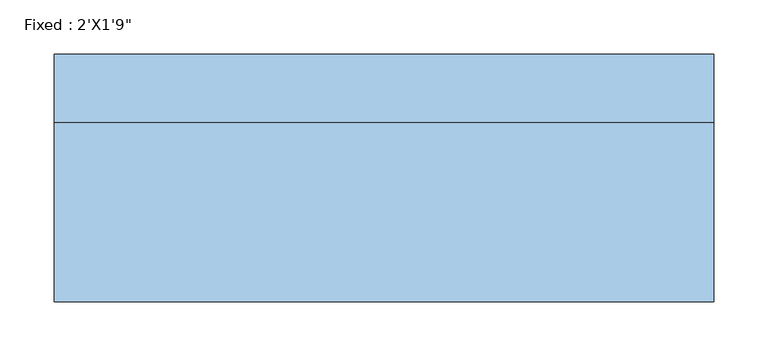
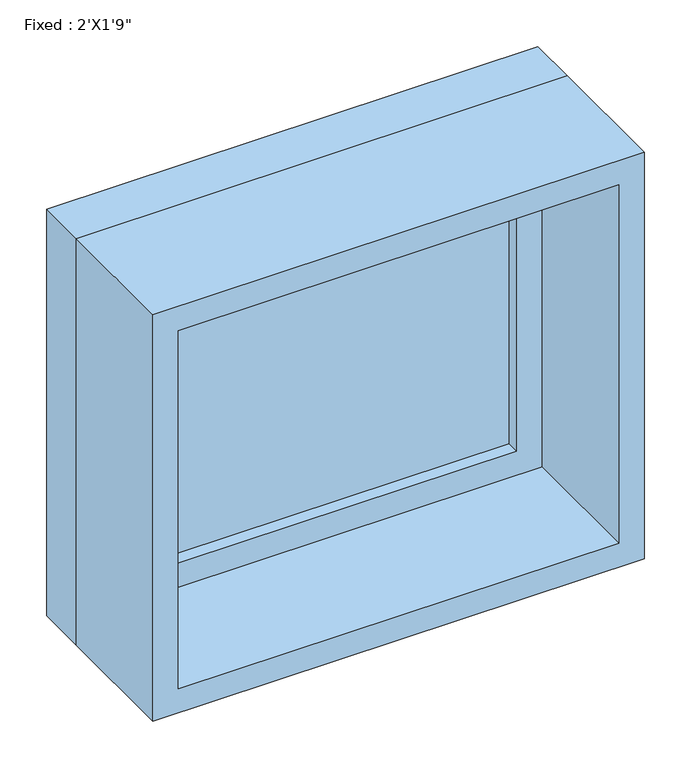
"""IFC4 building model written with IfcOpenShell, lengths in millimetres: window geometry."""

from ifc_helpers import new_model, si_unit, frame, origin, place, context, project, spatial, polyline, outline, extrude, source, transform, mapped, element, save


def window_9e637e28(model_context):
    return source(origin(), model_context, "Body", "SweptSolid", [
        extrude(outline(polyline([(203.2, 66.675), (-279.4, 66.675), (-279.4, 79.375), (203.2, 79.375), (203.2, 66.675)])), frame((0.0, 0.0, 2197.1), z_axis=(0.0, 0.0, 1.0), x_axis=(1.0, 0.0, 0.0)), (0.0, 0.0, 1.0), 406.4),
        extrude(outline(polyline([(2647.95, -323.85), (2152.65, -323.85), (2152.65, 247.65), (2647.95, 247.65), (2647.95, -323.85)]), holes=[polyline([(2603.5, -279.4), (2603.5, 203.2), (2197.1, 203.2), (2197.1, -279.4), (2603.5, -279.4)])]), frame((0.0, 50.8, 0.0), z_axis=(0.0, 1.0, 0.0), x_axis=(0.0, 0.0, 1.0)), (0.0, 0.0, 1.0), 44.45),
        extrude(outline(polyline([(2667.0, -342.9), (2133.6, -342.9), (2133.6, 266.7), (2667.0, 266.7), (2667.0, -342.9)]), holes=[polyline([(2635.25, -311.15), (2635.25, 234.95), (2165.35, 234.95), (2165.35, -311.15), (2635.25, -311.15)])]), frame((0.0, -114.3, 0.0), z_axis=(0.0, 1.0, 0.0), x_axis=(0.0, 0.0, 1.0)), (0.0, 0.0, 1.0), 165.1),
        extrude(outline(polyline([(2667.0, 266.7), (2667.0, -342.9), (2133.6, -342.9), (2133.6, 266.7), (2667.0, 266.7)]), holes=[polyline([(2647.95, 247.65), (2152.65, 247.65), (2152.65, -323.85), (2647.95, -323.85), (2647.95, 247.65)])]), frame((0.0, 50.8, 0.0), z_axis=(0.0, 1.0, 0.0), x_axis=(0.0, 0.0, 1.0)), (0.0, 0.0, 1.0), 63.5),
    ])


if __name__ == "__main__":
    model = new_model("IFC4")
    model_context = context("Model", 3, world=origin())
    ifc_project = project(units=[si_unit("LENGTHUNIT", "METRE", prefix="MILLI")], contexts=[model_context])
    site = spatial("IfcSite", under=ifc_project)
    building = spatial("IfcBuilding", under=site)
    placement = place(None, origin())
    window_shape = window_9e637e28(model_context)
    element("IfcWindow", 1, ObjectType="Fixed : 2'X1'9\"", at=placement, inside=building, context=model_context, shape_type="MappedRepresentation", body=[
        mapped(window_shape, transform((0.0, 0.0, 0.0), x_axis=(1.0, 0.0, 0.0), y_axis=(0.0, 1.0, 0.0), z_axis=(0.0, 0.0, 1.0))),
    ])
    save(model, "model.ifc")

# Revit data of these elements
# Type "Fixed : 2'X1'9\""
#   Type Mark = "20"
#   Construction Type Id = "GSP4R"
#   Assembly Code = "B2020100"
#   Analytic Construction = "1/8 in Pilkington single glazing"
#   Visual Light Transmittance = 0.9
#   Solar Heat Gain Coefficient = 0.78
#   Heat Transfer Coefficient (U) = 0.6496 BTU/(h·ft²·°F)
#   Height = 1' - 9"
#   Default Sill Height = 7' - 0"
#   Width = 2' - 0"
#   Window Inset = 0' - 0 3/4"
#   Define Thermal Properties by = 1
#   Glass Pane Material = Glass
#   Sash Material = Sash
#   Wall Closure = (empty or 0)
# Element 1 (IfcWindow, "Fixed : 2'X1'9\"")
#   Materials on its faces: "Sash", "Glass"
# Materials
#   "Glass": class "Glass", colour RGB 0 128 192, transparency 0.75, Description = "Soda Lime Glass", Cost = 0
#   "Sash": class "Wood", colour RGB 224 178 126, transparency 0, Cost = 0
